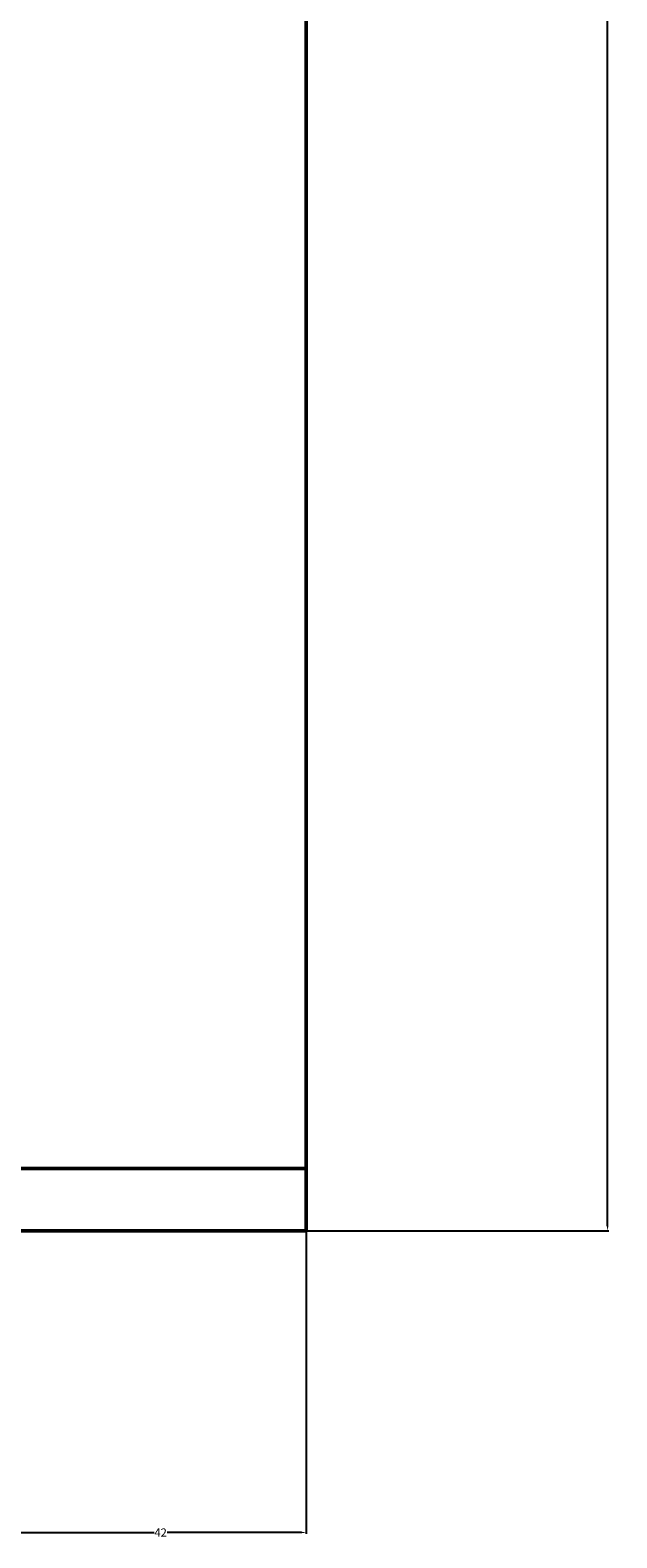
# Model space of a CAD drawing. Units: inches. Extents: x 3506 to 3958, y 1553 to 2506.
# Tile 6 of 16: x 3872 to 3957, y 1553 to 1770. Entities that reach past the tile are written whole.
import ezdxf

# ---------------------------------------------------------------- set-up
doc = ezdxf.new("R2010")
doc.units = ezdxf.units.IN
doc.header["$MEASUREMENT"] = 0
doc.layers.add('A-ANNO-DIMS', color=2, linetype='Continuous', lineweight=18)
doc.layers.add('A-WALL', color=7, linetype='Continuous', lineweight=50)
doc.layers.add('A-WALL-PATT', color=251, linetype='Continuous', lineweight=13, true_color=0x636466)
doc.styles.get("Standard").update_dxf_attribs({"font": 'arial.ttf'})
doc.dimstyles.get("Standard").update_dxf_attribs({"dimtxt": 1.18, "dimasz": 0.68, "dimexe": 0.18, "dimexo": 0.0625, "dimgap": 0.09, "dimtad": 0, "dimtih": 1, "dimtoh": 1, "dimdec": 1, "dimzin": 0, "dimdsep": 46, "dimlunit": 3, "dimtxsty": 'Standard', "dimcen": 0.09, "dimadec": 0, "dimazin": 0, "dimtfac": 1, "dimtdec": 1, "dimtofl": 0, "dimtmove": 0, "dimatfit": 3, "dimfxl": 1, "dimtolj": 1, "dimtzin": 0, "dimarcsym": 0})

# ---------------------------------------------------------------- blocks, each defined once
blk = doc.blocks.new('*D39')
at = {"layer": 'A-ANNO-DIMS', "color": 0, "lineweight": -2, "transparency": 16777216}
for p, q in [((3911.79, 2461.39), (3955.36, 2461.39)), ((3955.18, 2460.71), (3955.18, 2030.09)), ((3955.18, 1598.07), (3955.18, 2028.7)), ((3911.79, 1597.39), (3955.36, 1597.39))]:
    blk.add_line(p, q, dxfattribs=at)
at = {"layer": 'A-ANNO-DIMS', "color": 0, "transparency": 16777216}
for points in [[(3955.07, 2460.71), (3955.29, 2460.71), (3955.18, 2461.39)], [(3955.07, 1598.07), (3955.29, 1598.07), (3955.18, 1597.39)]]:
    blk.add_solid(points, dxfattribs=at)
at = {"layer": 'Defpoints', "color": 0, "transparency": 16777216}
for p in [(3911.73, 2461.39), (3955.18, 2461.39), (3911.73, 1597.39)]:
    blk.add_point(p, dxfattribs=at)
at = {"layer": 'A-ANNO-DIMS', "color": 0, "transparency": 16777216, "insert": (3955.18, 2029.39), "char_height": 1.18, "attachment_point": 5}
blk.add_mtext('\\A1;864', dxfattribs=at)
blk = doc.blocks.new('*D40')
at = {"layer": 'A-ANNO-DIMS', "color": 0, "lineweight": -2, "transparency": 16777216}
for p, q in [((3869.73, 1770.33), (3869.73, 1553.76)), ((3911.73, 1597.33), (3911.73, 1553.76)), ((3870.41, 1553.94), (3889.78, 1553.94)), ((3911.05, 1553.94), (3891.68, 1553.94))]:
    blk.add_line(p, q, dxfattribs=at)
at = {"layer": 'A-ANNO-DIMS', "color": 0, "transparency": 16777216}
for points in [[(3870.41, 1554.06), (3870.41, 1553.83), (3869.73, 1553.94)], [(3911.05, 1554.06), (3911.05, 1553.83), (3911.73, 1553.94)]]:
    blk.add_solid(points, dxfattribs=at)
at = {"layer": 'Defpoints', "color": 0, "transparency": 16777216}
for p in [(3869.73, 1770.39), (3911.73, 1597.39), (3911.73, 1553.94)]:
    blk.add_point(p, dxfattribs=at)
at = {"layer": 'A-ANNO-DIMS', "color": 0, "transparency": 16777216, "insert": (3890.73, 1553.94), "char_height": 1.18, "attachment_point": 5}
blk.add_mtext('\\A1;42', dxfattribs=at)

msp = doc.modelspace()

# ---------------------------------------------------------------- hatches: boundary and pattern name
at = {"layer": 'A-WALL-PATT'}
h = msp.add_hatch(dxfattribs=at)
h.set_pattern_fill('ANSI31', color=256)
h.paths.add_polyline_path([(3911.7302, 2461.3942), (3551.7302, 2461.3942), (3551.7302, 2152.516), (3560.7302, 2152.516), (3560.7302, 2116.516), (3551.7302, 2116.516), (3551.7302, 1920.5711), (3556.2302, 1920.5711), (3560.7302, 1920.5711), (3560.7302, 2000.3942), (3692.7302, 2000.3942), (3692.7302, 1997.3942), (3697.7302, 1997.3942), (3697.7302, 2000.3942), (3771.7302, 2000.3942), (3771.7302, 1997.3942), (3776.7302, 1997.3942), (3776.7302, 1997.7206), (3778.5802, 1997.7206), (3807.5802, 1997.7206), (3807.5802, 1996.4519), (3778.5802, 1996.4519), (3778.5802, 1997.7206), (3776.7302, 1997.7206), (3776.7302, 1997.3942), (3771.7302, 1997.3942), (3771.7302, 2000.3942), (3697.7302, 2000.3942), (3697.7302, 1997.3942), (3692.7302, 1997.3942), (3689.8302, 1997.3942), (3689.8302, 1995.8192), (3653.8302, 1995.8192), (3653.8302, 1997.3942), (3689.8302, 1997.3942), (3692.7302, 1997.3942), (3692.7302, 2000.3942), (3560.7302, 2000.3942), (3560.7302, 1920.5711), (3551.7302, 1920.5711), (3551.7302, 1884.5711), (3551.7302, 1597.3942), (3911.7302, 1597.3942)], flags=17)
h.paths.add_polyline_path([(3596.7302, 2005.3942), (3596.7302, 2057.3035, -0.38730371), (3569.1778, 2085), (3569.15, 2085), (3569.15, 2086.2688), (3598.15, 2086.2688), (3598.15, 2085), (3569.1778, 2085, 0.38730371), (3596.7302, 2057.3035), (3596.7302, 2057.3942), (3601.7302, 2057.3942), (3601.7302, 2055.3942), (3630.7302, 2055.3942), (3630.7302, 2034.3942), (3694.7302, 2034.3942), (3694.7302, 2053.3942), (3699.7302, 2053.3942), (3699.7302, 2005.3942), (3860.7302, 2005.3942), (3860.7302, 2173.3942), (3771.7302, 2173.3942), (3771.7302, 2194.3942), (3776.7302, 2194.3942), (3776.7302, 2178.3942), (3860.7302, 2178.3942), (3860.7302, 2231.3942), (3601.7302, 2231.3942), (3601.7302, 2241.426), (3596.7302, 2241.426), (3596.7302, 2231.3942), (3560.7302, 2231.3942), (3560.7302, 2315.3942), (3596.7302, 2315.3942), (3596.7302, 2312.3942), (3601.7302, 2312.3942), (3601.7302, 2315.3942), (3697.7302, 2315.3942), (3697.7302, 2413.3942), (3692.7302, 2413.3942), (3692.7302, 2320.3942), (3560.7302, 2320.3942), (3560.7302, 2452.3942), (3692.7302, 2452.3942), (3692.7302, 2449.3942), (3697.7302, 2449.3942), (3697.7302, 2452.3942), (3771.7302, 2452.3942), (3771.7302, 2449.3942), (3776.7302, 2449.3942), (3776.7302, 2452.3942), (3860.7302, 2452.3942), (3860.7302, 2437.2075), (3865.2302, 2437.2075), (3865.2302, 2413.2075), (3860.7302, 2413.2075), (3860.7302, 2367.6976), (3865.2302, 2367.6976), (3869.7302, 2367.6976), (3869.7302, 2319.6976), (3860.7302, 2319.6976), (3860.7302, 2211.6248), (3869.7302, 2211.6248), (3869.7302, 2187.6248), (3860.7302, 2187.6248), (3860.7302, 2138.4346), (3865.2302, 2138.4346), (3869.7302, 2138.4346), (3869.7302, 2090.4346), (3860.7302, 2090.4346), (3860.7302, 1985.8449), (3869.7302, 1985.8449), (3869.7302, 1961.8449), (3860.7302, 1961.8449), (3860.7302, 1897.0756), (3865.2302, 1897.0756), (3869.7302, 1897.0756), (3869.7302, 1849.0756), (3860.7302, 1849.0756), (3860.7302, 1847.8112), (3860.7302, 1779.3942), (3596.7302, 1779.3942), (3596.7302, 1831.3942), (3601.7302, 1831.3942), (3601.7302, 1828.3942), (3630.7302, 1828.3942), (3630.7302, 1808.3942), (3691.7302, 1808.3942), (3691.7302, 1815.3942), (3696.7302, 1815.3942), (3696.7302, 1779.3942), (3860.7302, 1779.3942), (3860.7302, 1947.3942), (3771.7302, 1947.3942), (3771.7302, 1968.3942), (3776.7302, 1968.3942), (3776.7302, 1952.3942), (3860.7302, 1952.3942), (3860.7302, 2005.3942)], flags=0)
h.paths.add_polyline_path([(3596.7302, 2038.8546), (3601.7302, 2038.8546), (3601.7302, 2014.8546), (3596.7302, 2014.8546)], flags=0)
h.paths.add_polyline_path([(3564.1688, 2107), (3564.1688, 2167), (3644.1688, 2167), (3644.1688, 2107)], flags=0)
h.paths.add_polyline_path([(3607.0972, 2052.0208), (3620.8472, 2052.0208, -0.41421356), (3621.9931, 2050.875), (3621.9931, 2025.6667, -0.41421356), (3620.8472, 2024.5208), (3607.0972, 2024.5208, -0.41421356), (3605.9514, 2025.6667), (3605.9514, 2050.875, -0.41421356)], flags=0)
h.paths.add_polyline_path([(3578.5688, 2115), (3565.3688, 2115), (3565.3688, 2135.8), (3578.5688, 2135.8), (3578.5688, 2138.2), (3565.3688, 2138.2), (3565.3688, 2159), (3580.5688, 2159), (3580.5688, 2153.8), (3593.7688, 2167), (3593.7688, 2151.8), (3578.5688, 2151.8)], flags=0)
h.paths.add_polyline_path([(3610.9167, 2050.875), (3620.0833, 2050.875, -0.41421356), (3620.8472, 2050.1111), (3620.8472, 2039.6076, -0.41421356), (3620.0833, 2038.8438), (3610.9167, 2038.8438, -0.41421356), (3610.1528, 2039.6076), (3610.1528, 2050.1111, -0.41421356)], flags=0)
h.paths.add_polyline_path([(3610.9167, 2037.6979), (3620.0833, 2037.6979, -0.41421356), (3620.8472, 2036.934), (3620.8472, 2026.4306, -0.41421356), (3620.0833, 2025.6667), (3610.9167, 2025.6667, -0.41421356), (3610.1528, 2026.4306), (3610.1528, 2036.934, -0.41421356)], flags=0)
h.paths.add_polyline_path([(3616.2639, 2044.7639, -1), (3614.7361, 2044.7639, -1)], flags=0)
h.paths.add_polyline_path([(3615.8819, 2044.7639, -1), (3615.1181, 2044.7639, -1)], flags=0)
h.paths.add_polyline_path([(3616.2639, 2031.7778, -1), (3614.7361, 2031.7778, -1)], flags=0)
h.paths.add_polyline_path([(3615.8819, 2031.7778, -1), (3615.1181, 2031.7778, -1)], flags=0)
h.paths.add_polyline_path([(3609.7539, 2021.7868), (3626.9586, 2021.7868), (3626.9586, 2008.8833), (3609.7539, 2008.8833)], flags=0)
h.paths.add_polyline_path([(3610.4708, 2021.07), (3621.2237, 2021.07), (3621.2237, 2009.6002), (3610.4708, 2009.6002)], flags=0)
h.paths.add_polyline_path([(3611.5461, 2019.9947), (3620.1484, 2019.9947), (3620.1484, 2010.6755), (3611.5461, 2010.6755)], flags=0)
h.paths.add_polyline_path([(3621.9405, 2021.07), (3626.2417, 2021.07), (3626.2417, 2009.6002), (3621.9405, 2009.6002)], flags=0)
h.paths.add_polyline_path([(3622.6574, 2020.3531), (3625.5248, 2020.3531), (3625.5248, 2017.4857), (3622.6574, 2017.4857)], flags=0)
h.paths.add_polyline_path([(3622.6574, 2016.7688), (3625.5248, 2016.7688), (3625.5248, 2010.317), (3622.6574, 2010.317)], flags=0)
h.paths.add_polyline_path([(3624.808, 2016.0519), (3624.808, 2013.9013), (3624.0911, 2013.9013), (3624.0911, 2013.1845), (3623.3743, 2013.1845), (3623.3743, 2013.9013), (3623.3743, 2016.0519)], flags=0)
h.paths.add_polyline_path([(3623.0158, 2012.8261), (3625.1664, 2012.8261), (3625.1664, 2012.1092), (3623.0158, 2012.1092)], flags=0)
h.paths.add_polyline_path([(3623.0158, 2011.7508), (3625.1664, 2011.7508), (3625.1664, 2011.0339), (3623.0158, 2011.0339)], flags=0)
h.paths.add_polyline_path([(3650.0591, 2031.8202), (3674.0368, 2031.8202), (3674.0368, 2012.638), (3669.2413, 2012.638), (3669.2413, 2011.8388), (3672.4383, 2011.8388), (3672.4383, 2011.0395), (3651.6576, 2011.0395), (3651.6576, 2011.8388), (3654.8546, 2011.8388), (3654.8546, 2012.638), (3650.0591, 2012.638)], flags=0)
h.paths.add_polyline_path([(3658.0517, 2024.6269, -1), (3651.6576, 2024.6269, -1)], flags=0)
h.paths.add_polyline_path([(3657.2524, 2024.6269, -1), (3652.4569, 2024.6269, -1)], flags=0)
h.paths.add_polyline_path([(3656.4532, 2024.6269, -1), (3653.2561, 2024.6269, -1)], flags=0)
h.paths.add_polyline_path([(3655.6539, 2024.6269, -1), (3654.0554, 2024.6269, -1)], flags=0)
h.paths.add_polyline_path([(3657.2524, 2017.4336, -1), (3652.4569, 2017.4336, -1)], flags=0)
h.paths.add_polyline_path([(3656.4532, 2017.4336, -1), (3653.2561, 2017.4336, -1)], flags=0)
h.paths.add_polyline_path([(3655.6539, 2017.4336, -1), (3654.0554, 2017.4336, -1)], flags=0)
h.paths.add_polyline_path([(3659.6502, 2027.8239), (3664.4457, 2027.8239), (3664.4457, 2015.0358), (3659.6502, 2015.0358)], flags=0)
h.paths.add_polyline_path([(3663.6465, 2027.0247), (3663.6465, 2015.8351), (3660.4494, 2015.8351), (3660.4494, 2027.0247)], flags=0)
h.paths.add_polyline_path([(3562.6688, 1945.5), (3642.6688, 1945.5), (3642.6688, 1885.5), (3562.6688, 1885.5)], flags=0)
h.paths.add_polyline_path([(3671.6391, 2024.6269, -1), (3666.8435, 2024.6269, -1)], flags=0)
h.paths.add_polyline_path([(3670.8398, 2024.6269, -1), (3667.6428, 2024.6269, -1)], flags=0)
h.paths.add_polyline_path([(3672.4383, 2017.4336, -1), (3666.0443, 2017.4336, -1)], flags=0)
h.paths.add_polyline_path([(3670.0405, 2024.6269, -1), (3668.442, 2024.6269, -1)], flags=0)
h.paths.add_polyline_path([(3671.6391, 2017.4336, -1), (3666.8435, 2017.4336, -1)], flags=0)
h.paths.add_polyline_path([(3670.8398, 2017.4336, -1), (3667.6428, 2017.4336, -1)], flags=0)
h.paths.add_polyline_path([(3592.2688, 1945.5), (3592.2688, 1930.3), (3577.0688, 1930.3), (3577.0688, 1893.5), (3563.8688, 1893.5), (3563.8688, 1914.3), (3577.0688, 1914.3), (3577.0688, 1916.7), (3563.8688, 1916.7), (3563.8688, 1937.5), (3579.0688, 1937.5), (3579.0688, 1932.3)], flags=0)
h.paths.add_polyline_path([(3670.0405, 2017.4336, -1), (3668.442, 2017.4336, -1)], flags=0)
h.paths.add_polyline_path([(3596.7302, 2283.3942), (3601.7302, 2283.3942), (3601.7302, 2265.426), (3599.2302, 2265.426), (3599.2302, 2241.426), (3596.7302, 2241.426), (3596.7302, 2265.426)], flags=0)
h.paths.add_polyline_path([(3596.7302, 1810.7006), (3601.7302, 1810.7006), (3601.7302, 1786.7006), (3596.7302, 1786.7006)], flags=0)
h.paths.add_polyline_path([(3560.7302, 1770.3942), (3738.7302, 1770.3942), (3738.7302, 1746.3942), (3738.7302, 1722.3942), (3748.7302, 1722.3942), (3748.7302, 1674.3942), (3560.7302, 1674.3942)], flags=0)
h.paths.add_polyline_path([(3728.7302, 1746.3942), (3728.7302, 1756.0642), (3738.7302, 1746.3942), (3728.7302, 1738.1582), (3728.7302, 1698.3942), (3591.2519, 1698.3942), (3591.2519, 1746.3942)], flags=0)
h.paths.add_polyline_path([(3771.7302, 2399.3942), (3771.7302, 2420.3942), (3776.7302, 2420.3942), (3776.7302, 2404.3942), (3776.7302, 2399.3942)], flags=0)
h.paths.add_polyline_path([(3911.7302, 2461.3942), (3551.7302, 2461.3942), (3551.7302, 2152.516), (3560.7302, 2152.516), (3560.7302, 2116.516), (3551.7302, 2116.516), (3551.7302, 1920.5711), (3560.7302, 1920.5711), (3560.7302, 2000.3942), (3692.7302, 2000.3942), (3692.7302, 1997.3942), (3697.7302, 1997.3942), (3697.7302, 2000.3942), (3771.7302, 2000.3942), (3771.7302, 1997.3942), (3776.7302, 1997.3942), (3776.7302, 1997.7206), (3778.5802, 1997.7206), (3807.5802, 1997.7206), (3807.5802, 1996.4519), (3778.5802, 1996.4519), (3778.5802, 1997.7206), (3776.7302, 1997.7206), (3776.7302, 1997.3942), (3771.7302, 1997.3942), (3771.7302, 2000.3942), (3697.7302, 2000.3942), (3697.7302, 1997.3942), (3692.7302, 1997.3942), (3689.8302, 1997.3942), (3689.8302, 1995.8192), (3653.8302, 1995.8192), (3653.8302, 1997.3942), (3689.8302, 1997.3942), (3692.7302, 1997.3942), (3692.7302, 2000.3942), (3560.7302, 2000.3942), (3560.7302, 1920.5711), (3551.7302, 1920.5711), (3551.7302, 1597.3942), (3911.7302, 1597.3942)], flags=17)

# ---------------------------------------------------------------- linework, layer by layer
at = {"layer": 'A-WALL'}
for q in [(3560.7302, 1606.3942), (3911.7302, 1606.3942)]:
    msp.add_line((3902.7302, 1606.3942), q, dxfattribs=at)
msp.add_lwpolyline([(3551.7302, 2461.3942), (3911.7302, 2461.3942), (3911.7302, 1597.3942), (3551.7302, 1597.3942)], close=True, dxfattribs=at)

# ---------------------------------------------------------------- dimensions: what is measured, and where the dimension line sits
at = {"layer": 'A-ANNO-DIMS'}
dim = msp.add_linear_dim(base=(3955.1802, 2461.3942), p1=(3911.7302, 1597.3942), p2=(3911.7302, 2461.3942), angle=90, dimstyle='Standard', override={"dimdec": 0, "dimlfac": 1, "dimrnd": 0, "dimzin": 0, "dimdsep": 46, "dimlunit": 2}, dxfattribs=at)
dim.commit()
dim.dimension.update_dxf_attribs({"geometry": '*D39', "text_midpoint": (3955.1802, 2029.3942)})
dim = msp.add_linear_dim(base=(3911.7302, 1553.9442), p1=(3869.7302, 1770.3942), p2=(3911.7302, 1597.3942), dimstyle='Standard', override={"dimdec": 0, "dimlfac": 1, "dimrnd": 0, "dimzin": 0, "dimdsep": 46, "dimlunit": 2}, dxfattribs=at)
dim.commit()
dim.dimension.update_dxf_attribs({"geometry": '*D40', "text_midpoint": (3890.7302, 1553.9442)})

doc.saveas('drawing.dxf')
